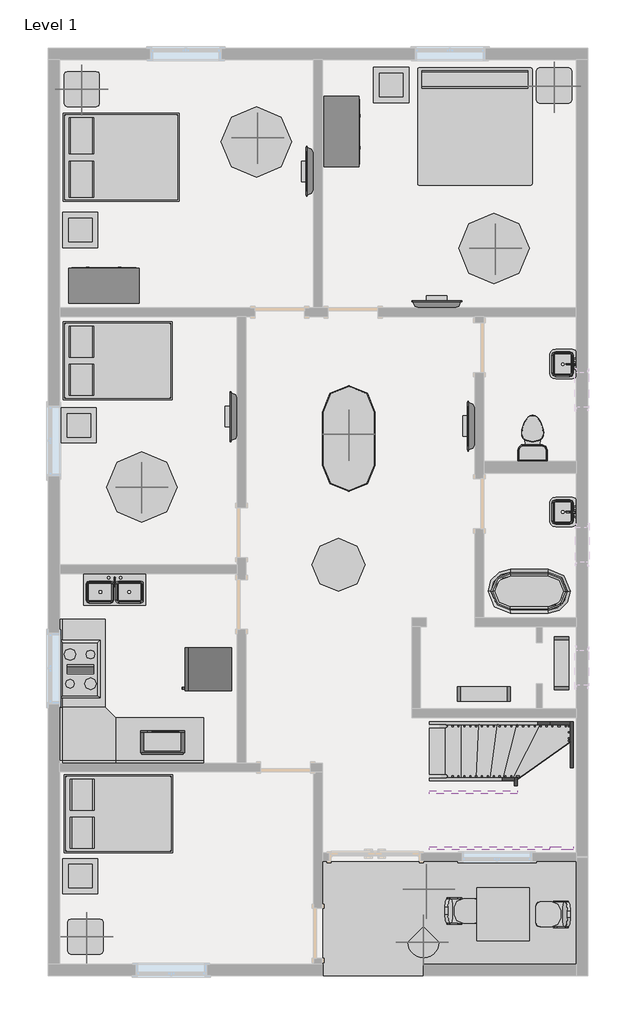
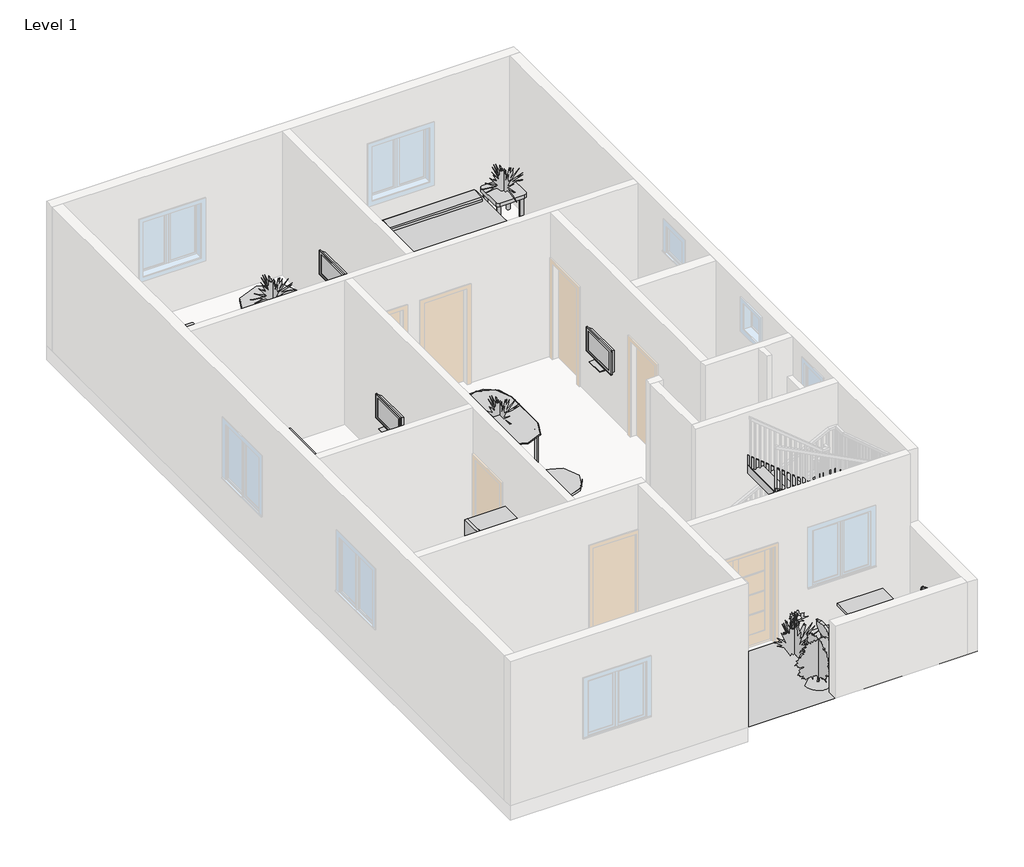
# One storey, part 3 of 3: 28 furniture elements, 9 geographic elements, 8 members, 7 flow terminals, 4 proxies, 1 stair flight.
"""IFC4 building model written with IfcOpenShell, lengths in millimetres."""

from ifc_helpers import new_model, si_unit, frame, origin, place, context, project, spatial, polyline, outline, extrude, triangles, transform, mapped, element, save
from components import proxy_bb1e6e30, proxy_8a8d5ab2, proxy_a13a33b2, flow_terminal_2b63360b, flow_terminal_a53be723, flow_terminal_62a433f7, toilet_domestic_3d_toilet_domestic_3d_f7549cf7, toilet_domestic_3d_toilet_domestic_3d_183bbd19, flow_terminal_a2f06f5b, furniture_c8abb964, furniture_1d2926bd, furniture_1fc5af50, furniture_9fa109b2, furniture_3d1d9cbc, furniture_417d203a, furniture_56245f3a, furniture_b5c51a22, furniture_2c34a4f9, furniture_905aceb5, furniture_c897acec, furniture_31d08a24, furniture_4d44e21c, furniture_356da175, rpc_plant_tropical_55f6ff97, rpc_plant_tropical_agave_1_5_93a2a214, rpc_plant_tropical_jungle_flame_3_9c4808c2, stair_flight_12d8a344

model = new_model("IFC4")

# Units and contexts
model_context = context("Model", 3, world=origin())
ifc_project = project(units=[si_unit("LENGTHUNIT", "METRE", prefix="MILLI")], contexts=[model_context])

# Site, building, storey
site = spatial("IfcSite", under=ifc_project)
building = spatial("IfcBuilding", under=site)
storey = spatial("IfcBuildingStorey", under=building, Name="Level 1", Elevation=0.0)

# Proxies
placement = place(None, origin())
element("IfcBuildingElementProxy", 1, Name="Building Element Proxy", at=placement, inside=storey, context=model_context, shape_type="Tessellation", body=[
    triangles([(-7495.2058731, -4647.4567314, 0.0), (-7495.2058731, -6628.6564407, 0.0), (-2897.80597, -6628.6564407, 0.0), (-2897.80597, -4558.5566345, 0.0)], [[1, 2, 3], [3, 4, 1]], closed=False),
])
proxy_shape = proxy_bb1e6e30(model_context)
element("IfcBuildingElementProxy", 2, Name="Cook Top-4 Unit : 36\" x 20\"", ObjectType="Cook Top-4 Unit : 36\" x 20\"", at=placement, inside=storey, context=model_context, shape_type="MappedRepresentation", body=[
    mapped(proxy_shape, transform((-11686.2060487, -1320.0567046, 0.0), x_axis=(0.0, 1.0000000000000002, 0.0), y_axis=(-1.0000000000000002, 0.0, 0.0), z_axis=(0.0, 0.0, 1.0))),
])
proxy_2_shape = proxy_8a8d5ab2(model_context)
element("IfcBuildingElementProxy", 3, Name="Microwave : 30\" x 16\" x 18\"", ObjectType="Microwave : 30\" x 16\" x 18\"", at=placement, inside=storey, context=model_context, shape_type="MappedRepresentation", body=[
    mapped(proxy_2_shape, transform((-9763.5131714, -2943.1372104, 0.0), x_axis=(-1.0000000000000004, 0.0, 0.0), y_axis=(0.0, -1.0000000000000004, 0.0), z_axis=(0.0, 0.0, 1.0))),
])
proxy_3_shape = proxy_a13a33b2(model_context)
element("IfcBuildingElementProxy", 4, Name="Refrigerator : 30\" x 32\" RH", ObjectType="Refrigerator : 30\" x 32\" RH", at=placement, inside=storey, context=model_context, shape_type="MappedRepresentation", body=[
    mapped(proxy_3_shape, transform((-9451.0060487, -1320.0567046, 0.0), x_axis=(0.0, -1.0000000000000004, 0.0), y_axis=(1.0000000000000004, 0.0, 0.0), z_axis=(0.0, 0.0, 1.0))),
])

# Flow terminals
flow_terminal_shape = flow_terminal_2b63360b(model_context)
element("IfcFlowTerminal", 5, ObjectType="Floor Drain - Rectangular : 5\"x5\" Strainer - 2\" Drain", at=placement, inside=storey, context=model_context, shape_type="MappedRepresentation", body=[
    mapped(flow_terminal_shape, transform((-3507.4060487, 3099.5432954, 0.0), x_axis=(1.0, 0.0, 0.0), y_axis=(0.0, 1.0, 0.0), z_axis=(0.0, 0.0, 1.0))),
])
element("IfcFlowTerminal", 6, ObjectType="Floor Drain - Rectangular : 5\"x5\" Strainer - 2\" Drain", at=placement, inside=storey, context=model_context, shape_type="MappedRepresentation", body=[
    mapped(flow_terminal_shape, transform((-3405.8060487, 597.6432954, 0.0), x_axis=(1.0, 0.0, 0.0), y_axis=(0.0, 1.0, 0.0), z_axis=(0.0, 0.0, 1.0))),
])
flow_terminal_2_shape = flow_terminal_a53be723(model_context)
element("IfcFlowTerminal", 7, ObjectType="Sink Kitchen-Double : 42\" x 21\"", at=placement, inside=storey, context=model_context, shape_type="MappedRepresentation", body=[
    mapped(flow_terminal_2_shape, transform((-11104.9952893, 49.1978943, 0.0), x_axis=(1.0, 0.0, 0.0), y_axis=(0.0, 1.0, 0.0), z_axis=(0.0, 0.0, 1.0))),
])
flow_terminal_3_shape = flow_terminal_62a433f7(model_context)
element("IfcFlowTerminal", 8, ObjectType="Sink Vanity-Square : 20\" x 18\"", at=placement, inside=storey, context=model_context, shape_type="MappedRepresentation", body=[
    mapped(flow_terminal_3_shape, transform((-3281.1514498, 1413.432536, 0.0), x_axis=(0.0, -1.0000000000000004, 0.0), y_axis=(1.0000000000000004, 0.0, 0.0), z_axis=(0.0, 0.0, 1.0))),
])
element("IfcFlowTerminal", 9, ObjectType="Sink Vanity-Square : 20\" x 18\"", at=placement, inside=storey, context=model_context, shape_type="MappedRepresentation", body=[
    mapped(flow_terminal_3_shape, transform((-3281.1514498, 3972.482536, 0.0), x_axis=(0.0, -1.0, 0.0), y_axis=(1.0, 0.0, 0.0), z_axis=(0.0, 0.0, 1.0))),
])
toilet_domestic_3d_toilet_domestic_3d_shape = toilet_domestic_3d_toilet_domestic_3d_f7549cf7(model_context)
toilet_domestic_3d_toilet_domestic_3d_2_shape = toilet_domestic_3d_toilet_domestic_3d_183bbd19(model_context)
element("IfcFlowTerminal", 10, ObjectType="Toilet-Domestic-3D : Toilet-Domestic-3D", at=placement, inside=storey, context=model_context, shape_type="MappedRepresentation", body=[
    mapped(toilet_domestic_3d_toilet_domestic_3d_shape, transform((-3855.0481236, 2768.7393228, 0.0), x_axis=(-1.0000000000000004, 0.0, 0.0), y_axis=(0.0, -1.0000000000000004, 0.0), z_axis=(0.0, 0.0, 1.0))),
    mapped(toilet_domestic_3d_toilet_domestic_3d_2_shape, transform((-3855.0481236, 2768.7393228, 0.0), x_axis=(-1.0000000000000004, 0.0, 0.0), y_axis=(0.0, -1.0000000000000004, 0.0), z_axis=(0.0, 0.0, 1.0))),
])
flow_terminal_4_shape = flow_terminal_a2f06f5b(model_context)
element("IfcFlowTerminal", 11, ObjectType="Tub-Free Standing-3D : 30\" x 60\"", at=placement, inside=storey, context=model_context, shape_type="MappedRepresentation", body=[
    mapped(flow_terminal_4_shape, transform((-3913.8060487, 26.1432954, 0.0), x_axis=(0.0, 1.0, 0.0), y_axis=(-1.0, 0.0, 0.0), z_axis=(0.0, 0.0, 1.0))),
])

# Furniture
furniture_shape = furniture_c8abb964(model_context)
element("IfcFurniture", 12, ObjectType="Bed-Box : Double 53\" x 74\"", at=placement, inside=storey, context=model_context, shape_type="MappedRepresentation", body=[
    mapped(furniture_shape, transform((-11272.9355569, 3674.7908364, 0.0), x_axis=(0.0, 1.0000000000000002, 0.0), y_axis=(-1.0000000000000002, 0.0, 0.0), z_axis=(0.0, 0.0, 1.0))),
])
element("IfcFurniture", 13, ObjectType="Bed-Box : Double 53\" x 74\"", at=placement, inside=storey, context=model_context, shape_type="MappedRepresentation", body=[
    mapped(furniture_shape, transform((-11260.2355569, -4161.1091636, 0.0), x_axis=(0.0, 1.0000000000000002, 0.0), y_axis=(-1.0000000000000002, 0.0, 0.0), z_axis=(0.0, 0.0, 1.0))),
])
furniture_2_shape = furniture_1d2926bd(model_context)
element("IfcFurniture", 14, ObjectType="Bed-Box : Queen 60\" x 79\"", at=placement, inside=storey, context=model_context, shape_type="MappedRepresentation", body=[
    mapped(furniture_2_shape, transform((-11209.4355569, 7192.6908364, 0.0), x_axis=(0.0, 1.0000000000000002, 0.0), y_axis=(-1.0000000000000002, 0.0, 0.0), z_axis=(0.0, 0.0, 1.0))),
])
furniture_3_shape = furniture_1fc5af50(model_context)
element("IfcFurniture", 15, ObjectType="Bed-Standard.0001 : King 78\" x 80\"", at=placement, inside=storey, context=model_context, shape_type="MappedRepresentation", body=[
    mapped(furniture_3_shape, transform((-5125.0945733, 8110.8383774, 0.0), x_axis=(1.0, 0.0, 0.0), y_axis=(0.0, 1.0, 0.0), z_axis=(0.0, 0.0, 1.0))),
])
furniture_4_shape = furniture_9fa109b2(model_context)
element("IfcFurniture", 16, ObjectType="Dresser : 48\" x 72\" x 24\"", at=placement, inside=storey, context=model_context, shape_type="MappedRepresentation", body=[
    mapped(furniture_4_shape, transform((-11548.9993086, 4946.1803413, 0.0), x_axis=(-1.0000000000000004, 0.0, 0.0), y_axis=(0.0, -1.0000000000000004, 0.0), z_axis=(0.0, 0.0, 1.0))),
])
element("IfcFurniture", 17, ObjectType="Dresser : 48\" x 72\" x 24\"", at=placement, inside=storey, context=model_context, shape_type="MappedRepresentation", body=[
    mapped(furniture_4_shape, transform((-7528.1690028, 8245.5365553, 0.0), x_axis=(0.0, 1.0000000000000002, 0.0), y_axis=(-1.0000000000000002, 0.0, 0.0), z_axis=(0.0, 0.0, 1.0))),
])
furniture_5_shape = furniture_3d1d9cbc(model_context)
element("IfcFurniture", 18, ObjectType="Seating-Auditorium : 18\" x 24\" x 30\"", at=placement, inside=storey, context=model_context, shape_type="MappedRepresentation", body=[
    mapped(furniture_5_shape, transform((-5272.0814586, -5343.9788357, 0.0), x_axis=(0.0, -1.0000000000000007, 0.0), y_axis=(1.0000000000000007, 0.0, 0.0), z_axis=(0.0, 0.0, 1.0))),
])
element("IfcFurniture", 19, ObjectType="Seating-Auditorium : 18\" x 24\" x 30\"", at=placement, inside=storey, context=model_context, shape_type="MappedRepresentation", body=[
    mapped(furniture_5_shape, transform((-3304.8306389, -5722.5845734, 0.0), x_axis=(0.0, 1.0000000000000002, 0.0), y_axis=(-1.0000000000000002, 0.0, 0.0), z_axis=(0.0, 0.0, 1.0))),
])
furniture_6_shape = furniture_417d203a(model_context)
element("IfcFurniture", 20, ObjectType="Shelving : 36\" x 10\" x 72\"", at=placement, inside=storey, context=model_context, shape_type="MappedRepresentation", body=[
    mapped(furniture_6_shape, transform((-3659.8060487, -1218.4567046, 0.0), x_axis=(0.0, 1.0, 0.0), y_axis=(-1.0, 0.0, 0.0), z_axis=(0.0, 0.0, 1.0))),
])
element("IfcFurniture", 21, ObjectType="Shelving : 36\" x 10\" x 72\"", at=placement, inside=storey, context=model_context, shape_type="MappedRepresentation", body=[
    mapped(furniture_6_shape, transform((-4701.2060487, -1447.0567046, 0.0), x_axis=(1.0, 0.0, 0.0), y_axis=(0.0, 1.0, 0.0), z_axis=(0.0, 0.0, 1.0))),
])
furniture_7_shape = furniture_56245f3a(model_context)
element("IfcFurniture", 22, ObjectType="TV - Flat Screen : 32\"", at=placement, inside=storey, context=model_context, shape_type="MappedRepresentation", body=[
    mapped(furniture_7_shape, transform((-7706.1446724, 7286.5987813, 914.4), x_axis=(0.0, -1.0000000000000004, 0.0), y_axis=(1.0000000000000004, 0.0, 0.0), z_axis=(0.0, 0.0, 1.0))),
])
element("IfcFurniture", 23, ObjectType="TV - Flat Screen : 32\"", at=placement, inside=storey, context=model_context, shape_type="MappedRepresentation", body=[
    mapped(furniture_7_shape, transform((-5517.9505629, 4986.8819191, 914.4), x_axis=(-1.0000000000000004, 0.0, 0.0), y_axis=(0.0, -1.0000000000000004, 0.0), z_axis=(0.0, 0.0, 1.0))),
])
element("IfcFurniture", 24, ObjectType="TV - Flat Screen : 32\"", at=placement, inside=storey, context=model_context, shape_type="MappedRepresentation", body=[
    mapped(furniture_7_shape, transform((-9026.9446724, 3044.7987813, 914.4), x_axis=(0.0, -1.0000000000000004, 0.0), y_axis=(1.0000000000000004, 0.0, 0.0), z_axis=(0.0, 0.0, 1.0))),
])
element("IfcFurniture", 25, ObjectType="TV - Flat Screen : 32\"", at=placement, inside=storey, context=model_context, shape_type="MappedRepresentation", body=[
    mapped(furniture_7_shape, transform((-4912.1446724, 2879.6987813, 990.6), x_axis=(0.0, -1.0000000000000002, 0.0), y_axis=(1.0000000000000002, 0.0, 0.0), z_axis=(0.0, 0.0, 1.0))),
])
furniture_8_shape = furniture_b5c51a22(model_context)
element("IfcFurniture", 26, ObjectType="Table-Coffee : 24\" x 24\" x 24\"", at=placement, inside=storey, context=model_context, shape_type="MappedRepresentation", body=[
    mapped(furniture_8_shape, transform((-11704.4718154, 6179.3322176, 0.0), x_axis=(1.0, 0.0, 0.0), y_axis=(0.0, 1.0, 0.0), z_axis=(0.0, 0.0, 1.0))),
])
element("IfcFurniture", 27, ObjectType="Table-Coffee : 24\" x 24\" x 24\"", at=placement, inside=storey, context=model_context, shape_type="MappedRepresentation", body=[
    mapped(furniture_8_shape, transform((-6319.6718154, 8687.5822176, 0.0), x_axis=(1.0, 0.0, 0.0), y_axis=(0.0, 1.0, 0.0), z_axis=(0.0, 0.0, 1.0))),
])
element("IfcFurniture", 28, ObjectType="Table-Coffee : 24\" x 24\" x 24\"", at=placement, inside=storey, context=model_context, shape_type="MappedRepresentation", body=[
    mapped(furniture_8_shape, transform((-11729.8718154, 2801.1322176, 0.0), x_axis=(1.0, 0.0, 0.0), y_axis=(0.0, 1.0, 0.0), z_axis=(0.0, 0.0, 1.0))),
])
element("IfcFurniture", 29, ObjectType="Table-Coffee : 24\" x 24\" x 24\"", at=placement, inside=storey, context=model_context, shape_type="MappedRepresentation", body=[
    mapped(furniture_8_shape, transform((-11704.4718154, -4996.6677824, 0.0), x_axis=(1.0, 0.0, 0.0), y_axis=(0.0, 1.0, 0.0), z_axis=(0.0, 0.0, 1.0))),
])
furniture_9_shape = furniture_2c34a4f9(model_context)
element("IfcFurniture", 30, ObjectType="Table-Dining Oval : 36\" x 72\"", at=placement, inside=storey, context=model_context, shape_type="MappedRepresentation", body=[
    mapped(furniture_9_shape, transform((-7396.1044094, 3069.5629676, 0.0), x_axis=(0.0, 1.0, 0.0), y_axis=(-1.0, 0.0, 0.0), z_axis=(0.0, 0.0, 1.0))),
])
furniture_10_shape = furniture_905aceb5(model_context)
element("IfcFurniture", 31, ObjectType="Table-Dining Round w Chairs : 36\" Diameter", at=placement, inside=storey, context=model_context, shape_type="MappedRepresentation", body=[
    mapped(furniture_10_shape, transform((-7319.4880159, 668.221984, 0.0), x_axis=(1.0, 0.0, 0.0), y_axis=(0.0, 1.0, 0.0), z_axis=(0.0, 0.0, 1.0))),
])
furniture_11_shape = furniture_c897acec(model_context)
element("IfcFurniture", 32, ObjectType="Table-Ellipse : 60\" x 48\"", at=placement, inside=storey, context=model_context, shape_type="MappedRepresentation", body=[
    mapped(furniture_11_shape, transform((-8638.2060487, 7798.5432954, 0.0), x_axis=(1.0, 0.0, 0.0), y_axis=(0.0, 1.0, 0.0), z_axis=(0.0, 0.0, 1.0))),
])
element("IfcFurniture", 33, ObjectType="Table-Ellipse : 60\" x 48\"", at=placement, inside=storey, context=model_context, shape_type="MappedRepresentation", body=[
    mapped(furniture_11_shape, transform((-4523.4060487, 5957.0432954, 0.0), x_axis=(0.0, 1.0000000000000002, 0.0), y_axis=(-1.0000000000000002, 0.0, 0.0), z_axis=(0.0, 0.0, 1.0))),
])
element("IfcFurniture", 34, ObjectType="Table-Ellipse : 60\" x 48\"", at=placement, inside=storey, context=model_context, shape_type="MappedRepresentation", body=[
    mapped(furniture_11_shape, transform((-10619.4060487, 1829.5432954, 0.0), x_axis=(0.0, 1.0000000000000002, 0.0), y_axis=(-1.0000000000000002, 0.0, 0.0), z_axis=(0.0, 0.0, 1.0))),
])
furniture_12_shape = furniture_31d08a24(model_context)
element("IfcFurniture", 35, ObjectType="Table-End : 24\" x 24\"", at=placement, inside=storey, context=model_context, shape_type="MappedRepresentation", body=[
    mapped(furniture_12_shape, transform((-11969.339679, 8560.5432954, 0.0), x_axis=(1.0, 0.0, 0.0), y_axis=(0.0, 1.0, 0.0), z_axis=(0.0, 0.0, 1.0))),
])
element("IfcFurniture", 36, ObjectType="Table-End : 24\" x 24\"", at=placement, inside=storey, context=model_context, shape_type="MappedRepresentation", body=[
    mapped(furniture_12_shape, transform((-3790.539679, 8624.0432954, 0.0), x_axis=(1.0, 0.0, 0.0), y_axis=(0.0, 1.0, 0.0), z_axis=(0.0, 0.0, 1.0))),
])
element("IfcFurniture", 37, ObjectType="Table-End : 24\" x 24\"", at=placement, inside=storey, context=model_context, shape_type="MappedRepresentation", body=[
    mapped(furniture_12_shape, transform((-11905.839679, -6101.6067046, 0.0), x_axis=(1.0, 0.0, 0.0), y_axis=(0.0, 1.0, 0.0), z_axis=(0.0, 0.0, 1.0))),
])
furniture_13_shape = furniture_4d44e21c(model_context)
element("IfcFurniture", 38, ObjectType="Table-Rectangular : 36\" x 36\"", at=placement, inside=storey, context=model_context, shape_type="MappedRepresentation", body=[
    mapped(furniture_13_shape, transform((-4364.6560487, -5561.8567046, 0.0), x_axis=(1.0, 0.0, 0.0), y_axis=(0.0, 1.0, 0.0), z_axis=(0.0, 0.0, 1.0))),
])
furniture_14_shape = furniture_356da175(model_context)
element("IfcFurniture", 39, ObjectType="Work Station Cubicle : 96\" x 96\"", at=placement, inside=storey, context=model_context, shape_type="MappedRepresentation", body=[
    mapped(furniture_14_shape, transform((-12536.8290564, -2813.9249523, 0.0), x_axis=(0.0, 1.0000000000000002, 0.0), y_axis=(-1.0000000000000002, 0.0, 0.0), z_axis=(0.0, 0.0, 1.0))),
])

# Geographic elements
rpc_plant_tropical_shape = rpc_plant_tropical_55f6ff97(model_context)
element("IfcGeographicElement", 40, ObjectType="RPC Plant - Tropical", at=placement, inside=storey, context=model_context, shape_type="MappedRepresentation", body=[
    mapped(rpc_plant_tropical_shape, transform((-5691.8060487, -5130.0567046, 0.0), x_axis=(1.0, 0.0, 0.0), y_axis=(0.0, 1.0, 0.0), z_axis=(0.0, 0.0, 1.0))),
])
rpc_plant_tropical_agave_1_5_shape = rpc_plant_tropical_agave_1_5_93a2a214(model_context)
element("IfcGeographicElement", 41, ObjectType="RPC Plant - Tropical : Agave - 1.5'", at=placement, inside=storey, context=model_context, shape_type="MappedRepresentation", body=[
    mapped(rpc_plant_tropical_agave_1_5_shape, transform((-11660.8060487, 8712.9432954, 609.6), x_axis=(1.0, 0.0, 0.0), y_axis=(0.0, 1.0, 0.0), z_axis=(0.0, 0.0, 1.0))),
])
element("IfcGeographicElement", 42, ObjectType="RPC Plant - Tropical : Agave - 1.5'", at=placement, inside=storey, context=model_context, shape_type="MappedRepresentation", body=[
    mapped(rpc_plant_tropical_agave_1_5_shape, transform((-8612.8060487, 7874.7432954, 609.6), x_axis=(1.0, 0.0, 0.0), y_axis=(0.0, 1.0, 0.0), z_axis=(0.0, 0.0, 1.0))),
])
element("IfcGeographicElement", 43, ObjectType="RPC Plant - Tropical : Agave - 1.5'", at=placement, inside=storey, context=model_context, shape_type="MappedRepresentation", body=[
    mapped(rpc_plant_tropical_agave_1_5_shape, transform((-3482.0060487, 8763.7432954, 609.6), x_axis=(1.0, 0.0, 0.0), y_axis=(0.0, 1.0, 0.0), z_axis=(0.0, 0.0, 1.0))),
])
element("IfcGeographicElement", 44, ObjectType="RPC Plant - Tropical : Agave - 1.5'", at=placement, inside=storey, context=model_context, shape_type="MappedRepresentation", body=[
    mapped(rpc_plant_tropical_agave_1_5_shape, transform((-4498.0060487, 5957.0432954, 609.6), x_axis=(1.0, 0.0, 0.0), y_axis=(0.0, 1.0, 0.0), z_axis=(0.0, 0.0, 1.0))),
])
element("IfcGeographicElement", 45, ObjectType="RPC Plant - Tropical : Agave - 1.5'", at=placement, inside=storey, context=model_context, shape_type="MappedRepresentation", body=[
    mapped(rpc_plant_tropical_agave_1_5_shape, transform((-10619.4060487, 1829.5432954, 609.6), x_axis=(1.0, 0.0, 0.0), y_axis=(0.0, 1.0, 0.0), z_axis=(0.0, 0.0, 1.0))),
])
element("IfcGeographicElement", 46, ObjectType="RPC Plant - Tropical : Agave - 1.5'", at=placement, inside=storey, context=model_context, shape_type="MappedRepresentation", body=[
    mapped(rpc_plant_tropical_agave_1_5_shape, transform((-7038.0060487, 2743.9432954, 609.6), x_axis=(1.0, 0.0, 0.0), y_axis=(0.0, 1.0, 0.0), z_axis=(0.0, 0.0, 1.0))),
])
element("IfcGeographicElement", 47, ObjectType="RPC Plant - Tropical : Agave - 1.5'", at=placement, inside=storey, context=model_context, shape_type="MappedRepresentation", body=[
    mapped(rpc_plant_tropical_agave_1_5_shape, transform((-11571.9060487, -5949.2067046, 609.6), x_axis=(1.0, 0.0, 0.0), y_axis=(0.0, 1.0, 0.0), z_axis=(0.0, 0.0, 1.0))),
])
rpc_plant_tropical_jungle_flame_3_shape = rpc_plant_tropical_jungle_flame_3_9c4808c2(model_context)
element("IfcGeographicElement", 48, ObjectType="RPC Plant - Tropical : Jungle Flame - 3'", at=placement, inside=storey, context=model_context, shape_type="MappedRepresentation", body=[
    mapped(rpc_plant_tropical_jungle_flame_3_shape, transform((-5742.6060487, -6044.4567046, 0.0), x_axis=(1.0, 0.0, 0.0), y_axis=(0.0, 1.0, 0.0), z_axis=(0.0, 0.0, 1.0))),
])

# Members
element("IfcMember", 49, ObjectType="Stringer - 2\" Width", at=placement, inside=storey, context=model_context, shape_type="SweptSolid", body=[
    extrude(outline(polyline([(229.639954, -5644.7377406), (0.0, -5644.7377406), (0.0, -5424.975423), (962.500629, -3557.3205489), (1305.3956453, -3557.3205489), (229.639954, -5644.7377406)])), frame((0.0, -2285.2567046, 0.0), z_axis=(0.0, 1.0, 0.0), x_axis=(0.0, 0.0, 1.0)), (0.0, 0.0, 1.0), 50.8),
])
element("IfcMember", 50, ObjectType="Stringer - 2\" Width", at=placement, inside=storey, context=model_context, shape_type="SweptSolid", body=[
    extrude(outline(polyline([(-3557.3205489, -2285.2567046), (-3557.3205489, -2234.4567046), (-3202.6060487, -2234.4567046), (-3202.6060487, -2285.2567046), (-3557.3205489, -2285.2567046)])), frame((0.0, 0.0, 962.500629), z_axis=(0.0, 0.0, 1.0), x_axis=(1.0, 0.0, 0.0)), (0.0, 0.0, 1.0), 342.8950162),
])
element("IfcMember", 51, ObjectType="Stringer - 2\" Width", at=placement, inside=storey, context=model_context, shape_type="SweptSolid", body=[
    extrude(outline(polyline([(-2234.4567046, 1289.0952212), (-2234.4567046, 1000.5956453), (-2403.9791875, 1000.5956453), (-4393.4567046, 1638.9682298), (-4393.4567046, 1969.9972697), (-4356.4765873, 1969.9972697), (-2234.4567046, 1289.0952212)])), frame((-3202.6060487, 0.0, 0.0), z_axis=(1.0, 0.0, 0.0), x_axis=(0.0, 1.0, 0.0)), (0.0, 0.0, 1.0), 50.8),
])
element("IfcMember", 52, ObjectType="Stringer - 2\" Width", at=placement, inside=storey, context=model_context, shape_type="SweptSolid", body=[
    extrude(outline(polyline([(-3151.8060487, -4393.4567046), (-3151.8060487, -4444.2567046), (-3557.3205489, -4444.2567046), (-3557.3205489, -4393.4567046), (-3151.8060487, -4393.4567046)])), frame((0.0, 0.0, 1649.8904473), z_axis=(0.0, 0.0, 1.0), x_axis=(1.0, 0.0, 0.0)), (0.0, 0.0, 1.0), 320.1068224),
])
element("IfcMember", 53, ObjectType="Stringer - 2\" Width", at=placement, inside=storey, context=model_context, shape_type="SweptSolid", body=[
    extrude(outline(polyline([(1649.8904473, -3557.3205489), (1969.9972697, -3557.3205489), (3045.7529609, -5644.7377406), (2725.6461385, -5644.7377406), (1649.8904473, -3557.3205489)])), frame((0.0, -4444.2567046, 0.0), z_axis=(0.0, 1.0, 0.0), x_axis=(0.0, 0.0, 1.0)), (0.0, 0.0, 1.0), 50.8),
])
element("IfcMember", 54, ObjectType="Stringer - 2\" Width", at=placement, inside=storey, context=model_context, shape_type="SweptSolid", body=[
    extrude(outline(polyline([(176.1764461, -5644.7377406), (0.0, -5644.7377406), (0.0, -5378.476096), (987.1410923, -4167.8060487), (1380.418648, -4167.8060487), (176.1764461, -5644.7377406)])), frame((0.0, -3250.4567046, 0.0), z_axis=(0.0, 1.0, 0.0), x_axis=(0.0, 0.0, 1.0)), (0.0, 0.0, 1.0), 50.8),
])
element("IfcMember", 55, ObjectType="Stringer - 2\" Width", at=placement, inside=storey, context=model_context, shape_type="SweptSolid", body=[
    extrude(outline(polyline([(-3199.6567046, 1573.2682978), (-3199.6567046, 1028.5617647), (-3233.8989219, 1028.5617647), (-3428.2567046, 1360.465107), (-3428.2567046, 1926.1409689), (-3406.293822, 1926.1409689), (-3199.6567046, 1573.2682978)])), frame((-4167.8060487, 0.0, 0.0), z_axis=(1.0, 0.0, 0.0), x_axis=(0.0, 1.0, 0.0)), (0.0, 0.0, 1.0), 50.8),
])
element("IfcMember", 56, ObjectType="Stringer - 2\" Width", at=placement, inside=storey, context=model_context, shape_type="SweptSolid", body=[
    extrude(outline(polyline([(1532.8634131, -4117.0060487), (1926.1409689, -4117.0060487), (3171.8038432, -5644.7377406), (2778.5262875, -5644.7377406), (1532.8634131, -4117.0060487)])), frame((0.0, -3479.0567046, 0.0), z_axis=(0.0, 1.0, 0.0), x_axis=(0.0, 0.0, 1.0)), (0.0, 0.0, 1.0), 50.8),
])

# Stair flight
stair_flight_shape = stair_flight_12d8a344(model_context)
element("IfcStairFlight", 57, ObjectType="2\" Tread 1\" Nosing 1/4\" Riser", at=placement, inside=storey, context=model_context, shape_type="MappedRepresentation", body=[
    mapped(stair_flight_shape, transform((0.0, 0.0, 0.0), x_axis=(1.0, 0.0, 0.0), y_axis=(0.0, 1.0, 0.0), z_axis=(0.0, 0.0, 1.0))),
])

save(model, "model.ifc")

# Revit data of these elements
# Type "Cook Top-4 Unit : 36\" x 20\""
#   Assembly Code = "E1090400"
#   Depth = 2' - 0"
#   Width = 3' - 0"
#   Burner Material = Steel, Chrome Plated
#   Cooktop Material = Steel, Polished
#   Default Elevation = 0
# Type "Microwave : 30\" x 16\" x 18\""
#   Assembly Code = "E1090400"
#   Depth = 1' - 4"
#   Height = 1' - 6"
#   Width = 2' - 6"
#   Microwave Material = Laminate, Ivory, Matte
#   Default Elevation = 0
# Type "Refrigerator : 30\" x 32\" RH"
#   Label = "REF."
#   Assembly Code = "E1090400"
#   Depth = 2' - 7 3/4"
#   Handle = 2' - 3"
#   Height = 5' - 10"
#   Rear Clearance = 0' - 2"
#   Top Door Height = 1' - 8"
#   Width = 2' - 5 3/8"
#   Material = Steel, Paint Finish, Ivory, Glossy
#   Default Elevation = 0
# Type "Floor Drain - Rectangular : 5\"x5\" Strainer - 2\" Drain"
#   WFU = 2
#   Strainer Height = 0' - 3 1/4"
#   Half Strainer Length = 0' - 2 1/2"
#   Strainer Length = 0' - 5"
#   Radius 2 = 0' - 3.04167"
#   Radius 1 = 0' - 2.02083"
#   Radius 3 = 0' - 2 1/32"
#   Pipe Radius = 1"
#   Pipe Diameter = 2"
#   Height 2 = 0' - 0.725"
#   Height 1 = 0' - 1 13/16"
#   Body Radius = 0' - 4 1/16"
#   Body Height = 0' - 3 5/8"
#   Body Diameter = 0' - 8 1/8"
#   Drain Material = none
#   HWFU = 0
#   Default Elevation = 0
#   CWFU = 0
# Type "Sink Kitchen-Double : 42\" x 21\""
#   Assembly Code = "D2010410"
#   Counter Height = 3' - 0"
#   Depth = 1' - 9"
#   Width = 3' - 6"
#   Faucet Material = Steel, Polished
#   Sink Material = Steel, Polished
#   Default Elevation = 0
# Type "Sink Vanity-Square : 20\" x 18\""
#   Assembly Code = "D2010400"
#   Counter Height = 2' - 7"
#   Depth = 1' - 6"
#   Width = 1' - 8"
#   Basin Material = Porcelain, Linen
#   Faucet Material = Steel, Polished
#   Default Elevation = 0
# Type "Toilet-Domestic-3D : Toilet-Domestic-3D"
#   Assembly Code = "D2010110"
#   Toilet - Bowl/Basin Material = Porcelain, Linen
#   Toilet - Seat Material = Laminate, Linen, Matte
#   Default Elevation = 0
# Type "Tub-Free Standing-3D : 30\" x 60\""
#   Assembly Code = "D2010110"
#   Height = 1' - 6"
#   Length = 4' - 8"
#   Width = 2' - 6"
#   Tub Material = Porcelain, Ivory
#   Default Elevation = 0
# Type "Bed-Box : Double 53\" x 74\""
#   Assembly Code = "E2020200"
#   Length = 6' - 2"
#   Width = 4' - 5"
#   Frame Material = Birch
#   Mattress Material = Cherry
#   Default Elevation = 0
# Type "Bed-Box : Queen 60\" x 79\""
#   Assembly Code = "E2020200"
#   Length = 6' - 7"
#   Width = 5' - 0"
#   Frame Material = Birch
#   Mattress Material = Cherry
#   Default Elevation = 0
# Type "Bed-Standard.0001 : King 78\" x 80\""
#   Assembly Code = "E2020200"
#   Length = 6' - 8"
#   Width = 6' - 6"
#   Leg Material = Steel, Chrome Plated
#   Mattress Material = Cherry
#   Default Elevation = 0
# Type "Dresser : 48\" x 72\" x 24\""
#   Assembly Code = "E2020200"
#   Depth = 2' - 0"
#   Height = 6' - 0"
#   Width = 4' - 0"
#   Dresser Material = Laminate - Ivory, Glossy
#   Drawer Material = Laminate, Ivory, Matte
#   Knob Material = Cherry
#   Default Elevation = 0
# Type "Seating-Auditorium : 18\" x 24\" x 30\""
#   Assembly Code = "E2020200"
#   Seat Material = Linen, Beige
#   Frame Material = Steel, Paint Finish, Dark Gray, Matte
#   Default Elevation = 0
# Type "Shelving : 36\" x 10\" x 72\""
#   Assembly Code = "E2020200"
#   Depth = 0' - 10"
#   Height = 6' - 0"
#   Width = 3' - 0"
#   Shelving Unit Material = Birch
#   Default Elevation = 0
# Type "TV - Flat Screen : 32\""
#   SinAng = 0' - 0.0193"
#   L = 2' - 3.79372"
#   H = 1' - 3.6354"
#   Thickness = 0' - 4.33071"
#   Diagonal = 2' - 7.88976"
#   CosAng = 0' - 0.03431"
#   Stand [instance default] = yes
#   Default Elevation = 0
# Type "Table-Coffee : 24\" x 24\" x 24\""
#   Assembly Code = "E2020200"
#   Height = 2' - 0"
#   Length = 2' - 0"
#   Width = 2' - 0"
#   Top Material = none
#   Frame Material = none
#   Default Elevation = 0
# Type "Table-Dining Oval : 36\" x 72\""
#   Assembly Code = "E2020200"
#   Length = 6' - 0"
#   Width = 3' - 0"
#   Base Material = Steel, Chrome Plated
#   Top Material = Glass - Clear, Grey
#   Default Elevation = 0
#   Description = (empty or 0)
# Type "Table-Dining Round w Chairs : 36\" Diameter"
#   Assembly Code = "E2020200"
#   Radius = 1' - 6"
#   Diameter = 3' - 0"
#   Height = 2' - 6"
#   Chairs = 4
#   Base Material = Pine
#   Top Material = Laminate, Linen, Matte
#   Default Elevation = 0
# Type "Table-Ellipse : 60\" x 48\""
#   Assembly Code = "E2020200"
#   Half Width = 2' - 0"
#   Half Length = 2' - 0"
#   Height = 2' - 0"
#   Length = 4' - 0"
#   Width = 4' - 0"
#   Base Material = Birch
#   Top Material = Birch
#   Default Elevation = 0
# Type "Table-End : 24\" x 24\""
#   Assembly Code = "E2020200"
#   Height = 2' - 0"
#   Length = 2' - 0"
#   Width = 2' - 0"
#   Base Material = Birch
#   Top Material = Laminate, Ivory, Matte
#   Default Elevation = 0
# Type "Table-Rectangular : 36\" x 36\""
#   Assembly Code = "E2020200"
#   Height = 2' - 6"
#   Length = 3' - 0"
#   Width = 3' - 0"
#   Base Material = Birch
#   Top Material = Copper
#   Default Elevation = 0
# Type "Work Station Cubicle : 96\" x 96\""
#   Assembly Code = "E2020"
#   Desktop Height = 2' - 6"
#   Desktop1 Width = 2' - 5"
#   Desktop2 Width = 2' - 5"
#   Panel Height = 2' - 6"
#   Panel1 Length = 5' - 0"
#   Panel2 Length = 5' - 0"
#   Cube Panel Material = Textile - Light Gray
#   Work Top Material = Laminate, Ivory, Matte
#   Default Elevation = 0
# Type "RPC Plant - Tropical"
#   built-in parameter 1005198 = "{2, 15},{39, RPC-16-FWM5-GM7X-C67P-4000-ST1L-LVER-AU},{1, 0},{1, 0},{2, 13},{1, 8},{5, Color},{1, 0},{1, 0},{3, 0.8},{3, 0.8},{3, 0.8},{1, 8},{7, BBoxMin},{1, 0},{1, 0},{1, 0},{1, 0},{1, 0},{1, 8},{7, BBoxMax},{1, 0},{1, 0},{1, 0},{1, 0},{1, 0},{2, 11},{9, RPCTypeId},{1, 0},{1, 0},{39, RPC-16-FWM5-GM7X-C67P-4000-ST1L-LVER-AU},{1, 6},{14, RPCPlantHeight},{1, 0},{1, 0},{1, 3},{2, 11},{7, keyword},{1, 0},{1, 0},{35, :RPCs:Shrubs [General]:Geometry:RPC},{2, 11},{8, category},{1, 0},{1, 0},{16, Shrubs [General]},{2, 11},{12, LocalizedUID},{1, 0},{1, 0},{10, Crane Lily},{2, 14},{6, Height},{1, 0},{1, 0},{1, 3},{1, 2},{16, Cast Reflections},{1, 0},{1, 0},{1, 0},{1, 2},{12, Cast Shadows},{1, 0},{1, 0},{1, 1},{1, 2},{9, Lock View},{1, 0},{1, 0},{1, 0},{1, 4},{5, ViewC},{1, 0},{1, 0},{1, 0},{21, assetlibrary_base.fbx},{1, 5},"
#   built-in parameter 1005195 = "RPC-16-FWM5-GM7X-C67P-4000-ST1L-LVER-AU"
#   Assembly Code = "G2050500"
#   Height = 3' - 0"
#   Default Elevation = 0
# Type "RPC Plant - Tropical : Agave - 1.5'"
#   built-in parameter 1005198 = "{2, 15},{39, RPC-16-G1GJ-63FX-7K5P-N000-ST1L-LVER-AU},{1, 0},{1, 0},{2, 13},{1, 8},{5, Color},{1, 0},{1, 0},{3, 0.8},{3, 0.8},{3, 0.8},{1, 8},{7, BBoxMin},{1, 0},{1, 0},{1, 0},{1, 0},{1, 0},{1, 8},{7, BBoxMax},{1, 0},{1, 0},{1, 0},{1, 0},{1, 0},{2, 11},{9, RPCTypeId},{1, 0},{1, 0},{39, RPC-16-G1GJ-63FX-7K5P-N000-ST1L-LVER-AU},{1, 6},{14, RPCPlantHeight},{1, 0},{1, 0},{3, 1.5},{2, 11},{7, keyword},{1, 0},{1, 0},{35, :RPCs:Plants [General]:Geometry:RPC},{2, 11},{8, category},{1, 0},{1, 0},{16, Plants [General]},{2, 11},{12, LocalizedUID},{1, 0},{1, 0},{5, Agave},{2, 14},{6, Height},{1, 0},{1, 0},{3, 1.5},{1, 2},{16, Cast Reflections},{1, 0},{1, 0},{1, 0},{1, 2},{12, Cast Shadows},{1, 0},{1, 0},{1, 1},{1, 2},{9, Lock View},{1, 0},{1, 0},{1, 0},{1, 4},{5, ViewC},{1, 0},{1, 0},{1, 0},{21, assetlibrary_base.fbx},{1, 5},"
#   built-in parameter 1005195 = "RPC-16-G1GJ-63FX-7K5P-N000-ST1L-LVER-AU"
#   Type Comments = "Agave"
#   Assembly Code = "G2050500"
#   Height = 1' - 6"
#   Default Elevation = 0
# Type "RPC Plant - Tropical : Jungle Flame - 3'"
#   built-in parameter 1005198 = "{2, 15},{39, RPC-16-FUVJ-JWG0-MWGK-8000-ST1L-LVER-AU},{1, 0},{1, 0},{2, 13},{1, 8},{5, Color},{1, 0},{1, 0},{3, 0.8},{3, 0.8},{3, 0.8},{1, 8},{7, BBoxMin},{1, 0},{1, 0},{1, 0},{1, 0},{1, 0},{1, 8},{7, BBoxMax},{1, 0},{1, 0},{1, 0},{1, 0},{1, 0},{2, 11},{9, RPCTypeId},{1, 0},{1, 0},{39, RPC-16-FUVJ-JWG0-MWGK-8000-ST1L-LVER-AU},{1, 6},{14, RPCPlantHeight},{1, 0},{1, 0},{1, 3},{2, 11},{7, keyword},{1, 0},{1, 0},{35, :RPCs:Shrubs [General]:Geometry:RPC},{2, 11},{8, category},{1, 0},{1, 0},{16, Shrubs [General]},{2, 11},{12, LocalizedUID},{1, 0},{1, 0},{12, Jungle Flame},{2, 14},{6, Height},{1, 0},{1, 0},{1, 3},{1, 2},{16, Cast Reflections},{1, 0},{1, 0},{1, 0},{1, 2},{12, Cast Shadows},{1, 0},{1, 0},{1, 1},{1, 2},{9, Lock View},{1, 0},{1, 0},{1, 0},{1, 4},{5, ViewC},{1, 0},{1, 0},{1, 0},{21, assetlibrary_base.fbx},{1, 5},"
#   built-in parameter 1005195 = "RPC-16-FUVJ-JWG0-MWGK-8000-ST1L-LVER-AU"
#   Type Comments = "Jungle Flame"
#   Assembly Code = "G2050500"
#   Height = 3' - 0"
#   Default Elevation = 0
# Element 1 (IfcBuildingElementProxy)
#   Material = none
#   Phase Created = New Construction
# Element 2 (IfcBuildingElementProxy, "Cook Top-4 Unit : 36\" x 20\"")
#   Phase Created = New Construction
#   Materials on its faces: "Steel, Chrome Plated", "Steel, Polished"
# Element 3 (IfcBuildingElementProxy, "Microwave : 30\" x 16\" x 18\"")
#   Phase Created = New Construction
#   Materials on its faces: "Laminate, Ivory, Matte", "Glass"
# Element 4 (IfcBuildingElementProxy, "Refrigerator : 30\" x 32\" RH")
#   Phase Created = New Construction
#   Materials on its faces: "Steel, Paint Finish, Ivory, Glossy", "Steel, Chrome Plated"
# Element 5 (IfcFlowTerminal, "Floor Drain - Rectangular : 5\"x5\" Strainer - 2\" Drain")
#   Mark = "5"
#   Phase Created = New Construction
# Element 6 (IfcFlowTerminal, "Floor Drain - Rectangular : 5\"x5\" Strainer - 2\" Drain")
#   Mark = "6"
#   Phase Created = New Construction
# Element 7 (IfcFlowTerminal, "Sink Kitchen-Double : 42\" x 21\"")
#   Mark = "8"
#   Phase Created = New Construction
#   Materials on its faces: "Steel, Polished"
# Element 8 (IfcFlowTerminal, "Sink Vanity-Square : 20\" x 18\"")
#   Mark = "3"
#   Phase Created = New Construction
#   Materials on its faces: "Porcelain, Linen", "Steel, Polished"
# Element 9 (IfcFlowTerminal, "Sink Vanity-Square : 20\" x 18\"")
#   Mark = "4"
#   Phase Created = New Construction
#   Materials on its faces: "Porcelain, Linen", "Steel, Polished"
# Element 10 (IfcFlowTerminal, "Toilet-Domestic-3D : Toilet-Domestic-3D")
#   Mark = "7"
#   Phase Created = New Construction
#   Materials on its faces: "Porcelain, Linen", "Laminate, Linen, Matte"
# Element 11 (IfcFlowTerminal, "Tub-Free Standing-3D : 30\" x 60\"")
#   Mark = "2"
#   Phase Created = New Construction
#   Materials on its faces: "Porcelain, Ivory"
# Elements 12, 13 (IfcFurniture, "Bed-Box : Double 53\" x 74\"")
#   Phase Created = New Construction
#   Materials on its faces: "Birch", "Cherry"
# Element 14 (IfcFurniture, "Bed-Box : Queen 60\" x 79\"")
#   Phase Created = New Construction
#   Materials on its faces: "Birch", "Cherry"
# Element 15 (IfcFurniture, "Bed-Standard.0001 : King 78\" x 80\"")
#   Phase Created = New Construction
#   Materials on its faces: "Linen, White", "Steel, Chrome Plated"
# Elements 16, 17 (IfcFurniture, "Dresser : 48\" x 72\" x 24\"")
#   Phase Created = New Construction
#   Materials on its faces: "Laminate, Ivory, Matte", "Cherry", "Laminate - Ivory, Glossy"
# Elements 18, 19 (IfcFurniture, "Seating-Auditorium : 18\" x 24\" x 30\"")
#   Phase Created = New Construction
#   Materials on its faces: "Steel, Paint Finish, Dark Gray, Matte", "Linen, Beige"
# Elements 20, 21 (IfcFurniture, "Shelving : 36\" x 10\" x 72\"")
#   Phase Created = New Construction
#   Materials on its faces: "Birch"
# Elements 22, 23, 24, 25 (IfcFurniture, "TV - Flat Screen : 32\"")
#   Stand = yes
#   Phase Created = New Construction
#   Materials on its faces: "TV - Black", "TV - Glass", "TV - Screen"
# Elements 26, 27, 28, 29 (IfcFurniture, "Table-Coffee : 24\" x 24\" x 24\"")
#   Phase Created = New Construction
#   Materials on its faces: "Glass - Clear, Grey"
# Element 30 (IfcFurniture, "Table-Dining Oval : 36\" x 72\"")
#   Phase Created = New Construction
#   Materials on its faces: "Steel, Chrome Plated", "Glass - Clear, Grey"
# Element 31 (IfcFurniture, "Table-Dining Round w Chairs : 36\" Diameter")
#   Phase Created = New Construction
#   Materials on its faces: "Pine", "Laminate, Linen, Matte"
# Elements 32, 33, 34 (IfcFurniture, "Table-Ellipse : 60\" x 48\"")
#   Phase Created = New Construction
#   Materials on its faces: "Birch"
# Elements 35, 36, 37 (IfcFurniture, "Table-End : 24\" x 24\"")
#   Phase Created = New Construction
#   Materials on its faces: "Laminate, Ivory, Matte", "Birch"
# Element 38 (IfcFurniture, "Table-Rectangular : 36\" x 36\"")
#   Phase Created = New Construction
#   Materials on its faces: "Birch", "Copper"
# Element 39 (IfcFurniture, "Work Station Cubicle : 96\" x 96\"")
#   Phase Created = New Construction
#   Materials on its faces: "Textile - Light Gray", "Laminate, Ivory, Matte"
# Element 40 (IfcGeographicElement, "RPC Plant - Tropical")
#   Phase Created = New Construction
# Elements 41, 42, 43, 44, 45, 46, 47 (IfcGeographicElement, "RPC Plant - Tropical : Agave - 1.5'")
#   Phase Created = New Construction
# Element 48 (IfcGeographicElement, "RPC Plant - Tropical : Jungle Flame - 3'")
#   Phase Created = New Construction
# Elements 49, 50, 51, 52, 53, 54, 55, 56 (IfcMember, "Stringer - 2\" Width")
#   Phase Created = New Construction
# Element 57 (IfcStairFlight, "2\" Tread 1\" Nosing 1/4\" Riser")
#   Phase Created = New Construction
# Materials
#   "Steel, Chrome Plated": class "Metal", colour RGB 17 17 17, transparency 0, Description = "Chromiuim plated steel", Cost = 0
#   "Steel, Polished": class "Metal", colour RGB 57 57 57, transparency 0, Description = "Polished steel", Cost = 0
#   "Laminate, Ivory, Matte": class "Plastic", colour RGB 247 247 239, transparency 0, Description = "Plastic Laminate - Ivory, Matte", Cost = 0
#   "Steel, Paint Finish, Ivory, Glossy": class "Metal", colour RGB 247 247 239, transparency 0, Description = "Steel, paint finish, ivory, glossy", Cost = 0
#   "Porcelain, Linen": class "Ceramic", colour RGB 249 239 230, transparency 0, Description = "Porcelain, linen", Cost = 0
#   "Laminate, Linen, Matte": class "Plastic", colour RGB 249 239 230, transparency 0, Description = "Plastic Laminate - Linen, Matte", Cost = 0
#   "Porcelain, Ivory": class "Ceramic", colour RGB 247 247 239, transparency 0, Description = "Porcelain, ivory", Cost = 0
#   "Birch": class "Wood", colour RGB 224 178 126, transparency 0, Description = "Betula Alleghaniensis", Cost = 0
#   "Cherry": class "Wood", colour RGB 226 177 128, transparency 0, Description = "Prunus Serotina", Cost = 0
#   "Laminate - Ivory, Glossy": colour RGB 247 247 239, transparency 0
#   "Linen, Beige": class "Textile", colour RGB 249 239 230, transparency 0, Description = "Linen, beige", Cost = 0
#   "Steel, Paint Finish, Dark Gray, Matte": class "Metal", colour RGB 0 0 0, transparency 0, Description = "Steel, paint finish, dark gray, matte", Cost = 0
#   "Glass - Clear, Grey": class "Glass", colour RGB 252 255 255, transparency 0.64
#   "Pine": class "Wood", colour RGB 223 192 134, transparency 0, Description = "Pinus Echinata", Cost = 0
#   "Copper": class "Metal", colour RGB 0 0 0, transparency 0, Description = "Copper, matte finish", Cost = 0
#   "Textile - Light Gray": class "Fabric", colour RGB 204 204 204, transparency 0
#   "Glass": class "Glass", colour RGB 0 128 192, transparency 0.75, Description = "Soda Lime Glass", Cost = 0
#   "Linen, White": class "Textile", colour RGB 247 247 239, transparency 0, Description = "Linen, white", Cost = 0
#   "TV - Black": colour RGB 49 49 49, transparency 0
#   "TV - Glass": colour RGB 157 157 157, transparency 0.9
#   "TV - Screen": colour RGB 0 0 0, transparency 0
